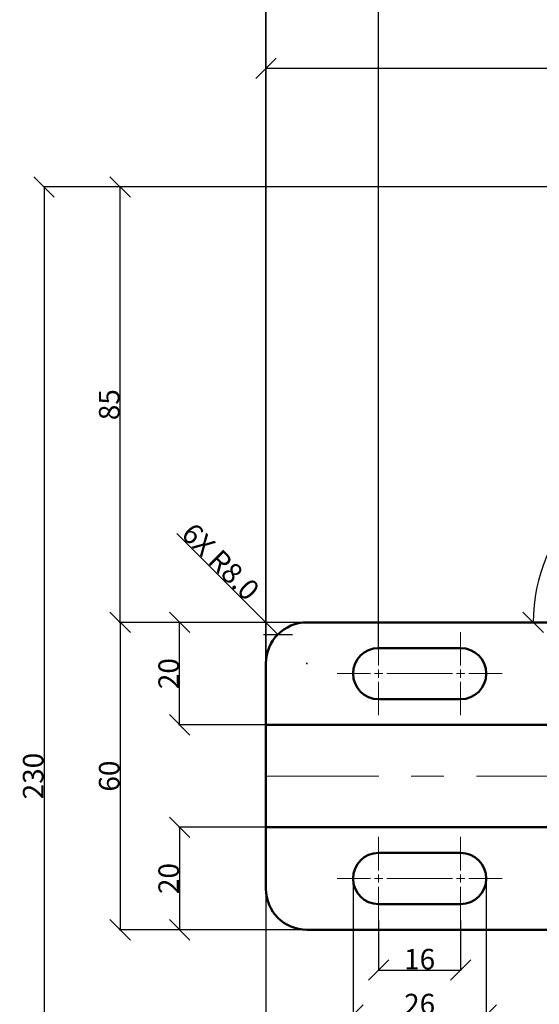
# Model space of a CAD drawing. Units: millimetres. Extents: x 263 to 611, y 50 to 522.
# Tile 2 of 5: x 263 to 364, y 157 to 349. Entities that reach past the tile are written whole.
import ezdxf

# ---------------------------------------------------------------- set-up
doc = ezdxf.new("R2010")
doc.units = ezdxf.units.MM
doc.header["$MEASUREMENT"] = 0
doc.linetypes.add('CENTER', pattern=[50.8, 31.75, -6.35, 6.35, -6.35])
for name, color, linetype, lineweight in [('M-CNTR', 1, 'CENTER', 18), ('M-DIMS', 2, 'Continuous', 25), ('M-OUTL', 7, 'Continuous', 50)]:
    doc.layers.add(name, color=color, linetype=linetype, lineweight=lineweight)
doc.styles.get("Standard").update_dxf_attribs({"font": 'arial.ttf'})
doc.dimstyles.get("Standard").update_dxf_attribs({"dimtxt": 4, "dimasz": 4, "dimexe": 0.18, "dimexo": 0.0625, "dimgap": 0.09, "dimtad": 1, "dimdec": 0, "dimzin": 0, "dimdsep": 46, "dimtxsty": 'Standard', "dimblk": 'OBLIQUE', "dimcen": 0.09, "dimclre": 251, "dimadec": 0, "dimazin": 0, "dimtfac": 1, "dimtdec": 0, "dimtofl": 0, "dimtmove": 0, "dimatfit": 3, "dimfxl": 1, "dimtolj": 1, "dimtzin": 0, "dimarcsym": 0})

# ---------------------------------------------------------------- blocks, each defined once
blk = doc.blocks.new('_Oblique')
at = {"color": 0, "linetype": 'ByBlock', "lineweight": -2}
blk.add_line((-0.5, -0.5), (0.5, 0.5), dxfattribs=at)
blk = doc.blocks.new('*D5')
at = {"layer": 'Defpoints', "color": 0, "transparency": 16777216}
for p in [(319.1, 231.08), (282.64, 171.08), (319.1, 171.08)]:
    blk.add_point(p, dxfattribs=at)
at = {"layer": 'M-DIMS', "color": 0, "lineweight": -2, "transparency": 16777216}
for p, q in [((319.04, 231.08), (282.46, 231.08)), ((282.64, 231.08), (282.64, 171.08)), ((319.04, 171.08), (282.46, 171.08))]:
    blk.add_line(p, q, dxfattribs=at)
at = {"layer": 'M-DIMS', "color": 0, "lineweight": -2, "transparency": 16777216, "xscale": 4, "yscale": 4, "zscale": 4}
for p, rotation in [((282.64, 231.08), 90), ((282.64, 171.08), 270)]:
    blk.add_blockref('_Oblique', p, dxfattribs=dict(at, rotation=rotation))
at = {"layer": 'M-DIMS', "color": 0, "transparency": 16777216, "insert": (280.51, 201.08), "char_height": 4, "attachment_point": 5, "rotation": 90}
blk.add_mtext('\\A1;60', dxfattribs=at)
blk = doc.blocks.new('*U6')
at = {"layer": 'M-CNTR', "color": 0, "transparency": 16777216}
for p, q in [((0, 1.6), (0, 8.12)), ((-8.12, 0), (-1.6, 0)), ((1.6, 0), (8.12, 0)), ((0, -8.12), (0, -1.6))]:
    blk.add_line(p, q, dxfattribs=at)
at = {"layer": 'M-CNTR', "color": 0, "linetype": 'Continuous', "transparency": 16777216}
for p, q in [((-0.8, 0), (0.8, 0)), ((0, -0.8), (0, 0.8))]:
    blk.add_line(p, q, dxfattribs=at)
blk = doc.blocks.new('*U7')
at = {"layer": 'M-CNTR', "color": 0, "transparency": 16777216}
for p, q in [((0, 1.6), (0, 8.12)), ((-8.12, 0), (-1.6, 0)), ((1.6, 0), (8.12, 0)), ((0, -8.12), (0, -1.6))]:
    blk.add_line(p, q, dxfattribs=at)
at = {"layer": 'M-CNTR', "color": 0, "linetype": 'Continuous', "transparency": 16777216}
for p, q in [((-0.8, 0), (0.8, 0)), ((0, -0.8), (0, 0.8))]:
    blk.add_line(p, q, dxfattribs=at)
blk = doc.blocks.new('*U8')
at = {"layer": 'M-CNTR', "color": 0, "transparency": 16777216}
for p, q in [((0, 1.6), (0, 8.12)), ((-8.12, 0), (-1.6, 0)), ((1.6, 0), (8.12, 0)), ((0, -8.12), (0, -1.6))]:
    blk.add_line(p, q, dxfattribs=at)
at = {"layer": 'M-CNTR', "color": 0, "linetype": 'Continuous', "transparency": 16777216}
for p, q in [((-0.8, 0), (0.8, 0)), ((0, -0.8), (0, 0.8))]:
    blk.add_line(p, q, dxfattribs=at)
blk = doc.blocks.new('*U9')
at = {"layer": 'M-CNTR', "color": 0, "transparency": 16777216}
for p, q in [((0, 1.6), (0, 8.12)), ((-8.12, 0), (-1.6, 0)), ((1.6, 0), (8.12, 0)), ((0, -8.12), (0, -1.6))]:
    blk.add_line(p, q, dxfattribs=at)
at = {"layer": 'M-CNTR', "color": 0, "linetype": 'Continuous', "transparency": 16777216}
for p, q in [((-0.8, 0), (0.8, 0)), ((0, -0.8), (0, 0.8))]:
    blk.add_line(p, q, dxfattribs=at)
blk = doc.blocks.new('*D18')
at = {"layer": 'Defpoints', "color": 0, "transparency": 16777216}
for p in [(546.1, 339.25), (546.1, 231.08), (311.1, 223.08)]:
    blk.add_point(p, dxfattribs=at)
at = {"layer": 'M-DIMS', "color": 0, "lineweight": -2, "transparency": 16777216}
for p, q in [((311.1, 223.14), (311.1, 339.43)), ((311.1, 339.25), (546.1, 339.25)), ((546.1, 231.14), (546.1, 339.43))]:
    blk.add_line(p, q, dxfattribs=at)
at = {"layer": 'M-DIMS', "color": 0, "lineweight": -2, "transparency": 16777216, "xscale": 4, "yscale": 4, "zscale": 4, "rotation": 180}
blk.add_blockref('_Oblique', (311.1, 339.25), dxfattribs=at)
at = {"layer": 'M-DIMS', "color": 0, "lineweight": -2, "transparency": 16777216, "xscale": 4, "yscale": 4, "zscale": 4}
blk.add_blockref('_Oblique', (546.1, 339.25), dxfattribs=at)
at = {"layer": 'M-DIMS', "color": 0, "transparency": 16777216, "insert": (428.6, 341.39), "char_height": 4, "attachment_point": 5}
blk.add_mtext('\\A1;235', dxfattribs=at)
blk = doc.blocks.new('*D19')
at = {"layer": 'Defpoints', "color": 0, "transparency": 16777216}
for p in [(294.25, 231.08), (319.1, 231.08), (311.1, 211.08)]:
    blk.add_point(p, dxfattribs=at)
at = {"layer": 'M-DIMS', "color": 0, "lineweight": -2, "transparency": 16777216}
for p, q in [((319.04, 231.08), (294.07, 231.08)), ((294.25, 211.08), (294.25, 231.08)), ((311.04, 211.08), (294.07, 211.08))]:
    blk.add_line(p, q, dxfattribs=at)
at = {"layer": 'M-DIMS', "color": 0, "lineweight": -2, "transparency": 16777216, "xscale": 4, "yscale": 4, "zscale": 4}
for p, rotation in [((294.25, 231.08), 90), ((294.25, 211.08), 270)]:
    blk.add_blockref('_Oblique', p, dxfattribs=dict(at, rotation=rotation))
at = {"layer": 'M-DIMS', "color": 0, "transparency": 16777216, "insert": (292.12, 221.08), "char_height": 4, "attachment_point": 5, "rotation": 90}
blk.add_mtext('\\A1;20', dxfattribs=at)
blk = doc.blocks.new('*D20')
at = {"layer": 'Defpoints', "color": 0, "transparency": 16777216}
for p in [(311.1, 191.08), (294.25, 171.08), (319.1, 171.08)]:
    blk.add_point(p, dxfattribs=at)
at = {"layer": 'M-DIMS', "color": 0, "lineweight": -2, "transparency": 16777216}
for p, q in [((311.04, 191.08), (294.07, 191.08)), ((294.25, 191.08), (294.25, 171.08)), ((319.04, 171.08), (294.07, 171.08))]:
    blk.add_line(p, q, dxfattribs=at)
at = {"layer": 'M-DIMS', "color": 0, "lineweight": -2, "transparency": 16777216, "xscale": 4, "yscale": 4, "zscale": 4}
for p, rotation in [((294.25, 191.08), 90), ((294.25, 171.08), 270)]:
    blk.add_blockref('_Oblique', p, dxfattribs=dict(at, rotation=rotation))
at = {"layer": 'M-DIMS', "color": 0, "transparency": 16777216, "insert": (292.12, 181.08), "char_height": 4, "attachment_point": 5, "rotation": 90}
blk.add_mtext('\\A1;20', dxfattribs=at)
blk = doc.blocks.new('*D21')
at = {"layer": 'Defpoints', "color": 0, "transparency": 16777216}
for p in [(282.64, 316.08), (404.1, 316.08), (319.1, 231.08)]:
    blk.add_point(p, dxfattribs=at)
at = {"layer": 'M-DIMS', "color": 0, "lineweight": -2, "transparency": 16777216}
for p, q in [((404.04, 316.08), (282.46, 316.08)), ((282.64, 231.08), (282.64, 316.08)), ((319.04, 231.08), (282.46, 231.08))]:
    blk.add_line(p, q, dxfattribs=at)
at = {"layer": 'M-DIMS', "color": 0, "lineweight": -2, "transparency": 16777216, "xscale": 4, "yscale": 4, "zscale": 4}
for p, rotation in [((282.64, 316.08), 90), ((282.64, 231.08), 270)]:
    blk.add_blockref('_Oblique', p, dxfattribs=dict(at, rotation=rotation))
at = {"layer": 'M-DIMS', "color": 0, "transparency": 16777216, "insert": (280.51, 273.58), "char_height": 4, "attachment_point": 5, "rotation": 90}
blk.add_mtext('\\A1;85', dxfattribs=at)
blk = doc.blocks.new('*D22')
at = {"layer": 'Defpoints', "color": 0, "transparency": 16777216}
for p in [(404.1, 316.08), (267.8, 86.08), (404.1, 86.08)]:
    blk.add_point(p, dxfattribs=at)
at = {"layer": 'M-DIMS', "color": 0, "lineweight": -2, "transparency": 16777216}
for p, q in [((404.04, 316.08), (267.62, 316.08)), ((267.8, 316.08), (267.8, 86.08)), ((404.04, 86.08), (267.62, 86.08))]:
    blk.add_line(p, q, dxfattribs=at)
at = {"layer": 'M-DIMS', "color": 0, "lineweight": -2, "transparency": 16777216, "xscale": 4, "yscale": 4, "zscale": 4}
for p, rotation in [((267.8, 316.08), 90), ((267.8, 86.08), 270)]:
    blk.add_blockref('_Oblique', p, dxfattribs=dict(at, rotation=rotation))
at = {"layer": 'M-DIMS', "color": 0, "transparency": 16777216, "insert": (265.67, 201.08), "char_height": 4, "attachment_point": 5, "rotation": 90}
blk.add_mtext('\\A1;230', dxfattribs=at)
blk = doc.blocks.new('*D23')
at = {"layer": 'Defpoints', "color": 0, "transparency": 16777216}
for p in [(333.1, 172.96), (349.1, 172.96), (349.1, 163.22)]:
    blk.add_point(p, dxfattribs=at)
at = {"layer": 'M-DIMS', "color": 0, "lineweight": -2, "transparency": 16777216}
for p, q in [((333.1, 172.9), (333.1, 163.04)), ((349.1, 172.9), (349.1, 163.04)), ((333.1, 163.22), (349.1, 163.22))]:
    blk.add_line(p, q, dxfattribs=at)
at = {"layer": 'M-DIMS', "color": 0, "lineweight": -2, "transparency": 16777216, "xscale": 4, "yscale": 4, "zscale": 4, "rotation": 180}
blk.add_blockref('_Oblique', (333.1, 163.22), dxfattribs=at)
at = {"layer": 'M-DIMS', "color": 0, "lineweight": -2, "transparency": 16777216, "xscale": 4, "yscale": 4, "zscale": 4}
blk.add_blockref('_Oblique', (349.1, 163.22), dxfattribs=at)
at = {"layer": 'M-DIMS', "color": 0, "transparency": 16777216, "insert": (341.1, 165.35), "char_height": 4, "attachment_point": 5}
blk.add_mtext('\\A1;16', dxfattribs=at)
blk = doc.blocks.new('*D24')
at = {"layer": 'Defpoints', "color": 0, "transparency": 16777216}
for p in [(328.1, 181.08), (354.1, 181.08), (354.1, 154.45)]:
    blk.add_point(p, dxfattribs=at)
at = {"layer": 'M-DIMS', "color": 0, "lineweight": -2, "transparency": 16777216}
for p, q in [((328.1, 181.02), (328.1, 154.27)), ((354.1, 181.02), (354.1, 154.27)), ((328.1, 154.45), (354.1, 154.45))]:
    blk.add_line(p, q, dxfattribs=at)
at = {"layer": 'M-DIMS', "color": 0, "lineweight": -2, "transparency": 16777216, "xscale": 4, "yscale": 4, "zscale": 4, "rotation": 180}
blk.add_blockref('_Oblique', (328.1, 154.45), dxfattribs=at)
at = {"layer": 'M-DIMS', "color": 0, "lineweight": -2, "transparency": 16777216, "xscale": 4, "yscale": 4, "zscale": 4}
blk.add_blockref('_Oblique', (354.1, 154.45), dxfattribs=at)
at = {"layer": 'M-DIMS', "color": 0, "transparency": 16777216, "insert": (341.1, 156.58), "char_height": 4, "attachment_point": 5}
blk.add_mtext('\\A1;26', dxfattribs=at)
blk = doc.blocks.new('*D25')
at = {"layer": 'Defpoints', "color": 0, "transparency": 16777216}
for p in [(311.1, 201.08), (426.1, 201.08), (426.1, 140.57)]:
    blk.add_point(p, dxfattribs=at)
at = {"layer": 'M-DIMS', "color": 0, "lineweight": -2, "transparency": 16777216}
for p, q in [((311.1, 201.02), (311.1, 140.39)), ((426.1, 201.02), (426.1, 140.39)), ((311.1, 140.57), (426.1, 140.57))]:
    blk.add_line(p, q, dxfattribs=at)
at = {"layer": 'M-DIMS', "color": 0, "lineweight": -2, "transparency": 16777216, "xscale": 4, "yscale": 4, "zscale": 4, "rotation": 180}
blk.add_blockref('_Oblique', (311.1, 140.57), dxfattribs=at)
at = {"layer": 'M-DIMS', "color": 0, "lineweight": -2, "transparency": 16777216, "xscale": 4, "yscale": 4, "zscale": 4}
blk.add_blockref('_Oblique', (426.1, 140.57), dxfattribs=at)
at = {"layer": 'M-DIMS', "color": 0, "transparency": 16777216, "insert": (368.6, 142.7), "char_height": 4, "attachment_point": 5}
blk.add_mtext('\\A1;115', dxfattribs=at)
blk = doc.blocks.new('*D29')
at = {"layer": 'Defpoints', "color": 0, "transparency": 16777216}
for p in [(396.1, 308.08), (379.68, 259.52), (396.1, 247.18), (319.1, 231.08), (380, 231.08)]:
    blk.add_point(p, dxfattribs=at)
at = {"layer": 'M-DIMS', "color": 0, "lineweight": -2, "transparency": 16777216}
blk.add_arc((396.1, 231.08), 32.84, 90, 180, dxfattribs=at)
at = {"layer": 'M-DIMS', "color": 0, "lineweight": -2, "transparency": 16777216, "xscale": 4, "yscale": 4, "zscale": 4}
for p, rotation in [((396.1, 263.92), 359.9999999999999), ((363.26, 231.08), 269.9999999999999)]:
    blk.add_blockref('_Oblique', p, dxfattribs=dict(at, rotation=rotation))
at = {"layer": 'M-DIMS', "color": 0, "transparency": 16777216, "insert": (371.37, 255.81), "char_height": 4, "attachment_point": 5, "rotation": 45}
blk.add_mtext('\\A1;90°', dxfattribs=at)
blk = doc.blocks.new('SLOT-10x26')
for p, q in [((0, 5), (0, 21)), ((10, 5), (10, 21))]:
    blk.add_line(p, q)
for centre, start, end in [((5, 21), 0, 180), ((5, 5), 180, 0)]:
    blk.add_arc(centre, 5, start, end)
blk = doc.blocks.new('*D52')
at = {"layer": 'Defpoints', "color": 0, "transparency": 16777216}
for p in [(333.1, 517.18), (333.1, 226.08), (311.1, 223.08)]:
    blk.add_point(p, dxfattribs=at)
at = {"layer": 'M-DIMS', "color": 251, "lineweight": -2, "transparency": 16777216}
for p, q in [((311.1, 223.14), (311.1, 517.36)), ((333.1, 226.14), (333.1, 517.36))]:
    blk.add_line(p, q, dxfattribs=at)
at = {"layer": 'M-DIMS', "color": 0, "lineweight": -2, "transparency": 16777216}
blk.add_line((311.1, 517.18), (333.1, 517.18), dxfattribs=at)
at = {"layer": 'M-DIMS', "color": 0, "lineweight": -2, "transparency": 16777216, "xscale": 4, "yscale": 4, "zscale": 4, "rotation": 180}
blk.add_blockref('_Oblique', (311.1, 517.18), dxfattribs=at)
at = {"layer": 'M-DIMS', "color": 0, "lineweight": -2, "transparency": 16777216, "xscale": 4, "yscale": 4, "zscale": 4}
blk.add_blockref('_Oblique', (333.1, 517.18), dxfattribs=at)
at = {"layer": 'M-DIMS', "color": 0, "transparency": 16777216, "insert": (322.1, 519.31), "char_height": 4, "attachment_point": 5}
blk.add_mtext('\\A1;22.0', dxfattribs=at)
blk = doc.blocks.new('*D53')
at = {"layer": 'Defpoints', "color": 0, "transparency": 16777216}
for p in [(578.1, 423.27), (311.1, 383.27), (578.1, 52.26)]:
    blk.add_point(p, dxfattribs=at)
at = {"layer": 'M-DIMS', "color": 251, "lineweight": -2, "transparency": 16777216}
for p, q in [((578.1, 423.21), (578.1, 52.08)), ((311.1, 383.21), (311.1, 52.08))]:
    blk.add_line(p, q, dxfattribs=at)
at = {"layer": 'M-DIMS', "color": 0, "lineweight": -2, "transparency": 16777216}
blk.add_line((311.1, 52.26), (578.1, 52.26), dxfattribs=at)
at = {"layer": 'M-DIMS', "color": 0, "lineweight": -2, "transparency": 16777216, "xscale": 4, "yscale": 4, "zscale": 4, "rotation": 180}
blk.add_blockref('_Oblique', (311.1, 52.26), dxfattribs=at)
at = {"layer": 'M-DIMS', "color": 0, "lineweight": -2, "transparency": 16777216, "xscale": 4, "yscale": 4, "zscale": 4}
blk.add_blockref('_Oblique', (578.1, 52.26), dxfattribs=at)
at = {"layer": 'M-DIMS', "color": 0, "transparency": 16777216, "insert": (444.6, 54.39), "char_height": 4, "attachment_point": 5}
blk.add_mtext('\\A1;267.0', dxfattribs=at)
blk = doc.blocks.new('*D57')
at = {"layer": 'Defpoints', "color": 0, "transparency": 16777216}
for p in [(372.02, 403.27), (311.1, 383.27), (372.02, 52.26)]:
    blk.add_point(p, dxfattribs=at)
at = {"layer": 'M-DIMS', "color": 251, "lineweight": -2, "transparency": 16777216}
for p, q in [((372.02, 403.21), (372.02, 52.08)), ((311.1, 383.21), (311.1, 52.08))]:
    blk.add_line(p, q, dxfattribs=at)
at = {"layer": 'M-DIMS', "color": 0, "lineweight": -2, "transparency": 16777216}
blk.add_line((311.1, 52.26), (372.02, 52.26), dxfattribs=at)
at = {"layer": 'M-DIMS', "color": 0, "lineweight": -2, "transparency": 16777216, "xscale": 4, "yscale": 4, "zscale": 4, "rotation": 180}
blk.add_blockref('_Oblique', (311.1, 52.26), dxfattribs=at)
at = {"layer": 'M-DIMS', "color": 0, "lineweight": -2, "transparency": 16777216, "xscale": 4, "yscale": 4, "zscale": 4}
blk.add_blockref('_Oblique', (372.02, 52.26), dxfattribs=at)
at = {"layer": 'M-DIMS', "color": 0, "transparency": 16777216, "insert": (341.56, 54.39), "char_height": 4, "attachment_point": 5}
blk.add_mtext('\\A1;60.92', dxfattribs=at)
blk = doc.blocks.new('*D69')
at = {"layer": 'Defpoints', "color": 0, "transparency": 16777216}
for p in [(426.1, 201.08), (387.21, 162.19)]:
    blk.add_point(p, dxfattribs=at)
at = {"layer": 'M-DIMS', "color": 251, "lineweight": -2, "transparency": 16777216}
for p, q in [((426.01, 201.08), (426.19, 201.08)), ((426.1, 200.99), (426.1, 201.17))]:
    blk.add_line(p, q, dxfattribs=at)
at = {"layer": 'M-DIMS', "color": 0, "lineweight": -2, "transparency": 16777216}
blk.add_line((355.69, 130.68), (387.21, 162.19), dxfattribs=at)
at = {"layer": 'M-DIMS', "color": 0, "lineweight": -2, "transparency": 16777216, "xscale": 4, "yscale": 4, "zscale": 4, "rotation": 44.99977533015295}
blk.add_blockref('_Oblique', (387.21, 162.19), dxfattribs=at)
at = {"layer": 'M-DIMS', "color": 0, "transparency": 16777216, "insert": (362.37, 140.36), "char_height": 4, "attachment_point": 5, "rotation": 44.9998}
blk.add_mtext('\\A1;4X R55.0', dxfattribs=at)
blk = doc.blocks.new('*D80')
at = {"layer": 'Defpoints', "color": 0, "transparency": 16777216}
for p in [(313.44, 228.74), (319.1, 223.08)]:
    blk.add_point(p, dxfattribs=at)
at = {"layer": 'M-DIMS', "color": 0, "lineweight": -2, "transparency": 16777216}
blk.add_line((293.72, 248.46), (313.44, 228.74), dxfattribs=at)
at = {"layer": 'M-DIMS', "color": 251, "lineweight": -2, "transparency": 16777216}
for p, q in [((319.01, 223.08), (319.19, 223.08)), ((319.1, 222.99), (319.1, 223.17))]:
    blk.add_line(p, q, dxfattribs=at)
at = {"layer": 'M-DIMS', "color": 0, "lineweight": -2, "transparency": 16777216, "xscale": 4, "yscale": 4, "zscale": 4, "rotation": 315.001848461854}
blk.add_blockref('_Oblique', (313.44, 228.74), dxfattribs=at)
at = {"layer": 'M-DIMS', "color": 0, "transparency": 16777216, "insert": (302.26, 242.94), "char_height": 4, "attachment_point": 5, "rotation": 315.0018}
blk.add_mtext('\\A1;6X R8.0', dxfattribs=at)

msp = doc.modelspace()

# ---------------------------------------------------------------- linework, layer by layer
at = {"layer": 'M-CNTR'}
msp.add_line((587.1329, 201.0815), (311.0988, 201.0815), dxfattribs=at)
at = {"layer": 'M-OUTL'}
for p, q in [((319.0988, 231.0815), (380.0011, 231.0815)), ((311.0988, 179.0815), (311.0988, 223.0815)), ((311.0988, 211.0815), (372.0156, 211.0815)), ((311.0988, 191.0815), (372.0156, 191.0815)), ((319.0988, 171.0815), (380.0011, 171.0815))]:
    msp.add_line(p, q, dxfattribs=at)
for centre, start, end in [((319.0988, 223.0815), 90, 180), ((319.0988, 179.0815), 180, 270)]:
    msp.add_arc(centre, 8, start, end, dxfattribs=at)

# ---------------------------------------------------------------- block references
at = {"layer": 'M-CNTR'}
for name, p in [('*U6', (333.0988, 221.0815)), ('*U7', (349.0988, 221.0815)), ('*U8', (333.0988, 181.0815)), ('*U9', (349.0988, 181.0815))]:
    msp.add_blockref(name, p, dxfattribs=at)
at = {"layer": 'M-OUTL'}
for p, rotation in [((328.0993, 226.0814), 269.9999999999999), ((328.0993, 186.0814), 269.9999999999998)]:
    msp.add_blockref('SLOT-10x26', p, dxfattribs=dict(at, rotation=rotation))

# ---------------------------------------------------------------- dimensions: what is measured, and where the dimension line sits
at = {"layer": 'M-DIMS'}
for base, p1, p2, override, picture, middle in [((333.0988, 517.1806), (311.0988, 223.0815), (333.0988, 226.0815), {"dimdec": 1, "dimlfac": 1, "dimrnd": 0, "dimzin": 0, "dimdsep": 46, "dimlunit": 2}, '*D52', (322.0988, 519.3128)), ((578.0988, 52.2557), (311.0988, 383.2727), (578.0988, 423.2727), {"dimdec": 1, "dimlfac": 1, "dimrnd": 0, "dimzin": 0, "dimdsep": 46, "dimlunit": 2}, '*D53', (444.5988, 54.388)), ((372.0156, 52.2557), (311.0988, 383.2727), (372.0156, 403.2727), {"dimdec": 2, "dimlfac": 1, "dimrnd": 0, "dimzin": 0, "dimdsep": 46, "dimlunit": 2}, '*D57', (341.5572, 54.388)), ((546.0988, 339.2528), (311.0988, 223.0815), (546.0988, 231.0815), {"dimclrd": 0, "dimclre": 0, "dimclrt": 0}, '*D18', (428.5988, 341.3864)), ((426.0988, 140.5664), (311.0988, 201.0815), (426.0988, 201.0815), {"dimclrd": 0, "dimclre": 0, "dimclrt": 0}, '*D25', (368.5988, 142.6987)), ((354.0988, 154.4515), (328.0988, 181.0815), (354.0988, 181.0815), {"dimclrd": 0, "dimclre": 0, "dimclrt": 0}, '*D24', (341.0988, 156.5838)), ((349.0988, 163.215), (333.0988, 172.9615), (349.0988, 172.9615), {"dimclrd": 0, "dimclre": 0, "dimclrt": 0}, '*D23', (341.0988, 165.3473))]:
    dim = msp.add_linear_dim(base=base, p1=p1, p2=p2, dimstyle='Standard', override=override, dxfattribs=at)
    dim.commit()
    dim.dimension.update_dxf_attribs({"geometry": picture, "text_midpoint": middle})
for base, p1, p2, picture, middle in [((267.7992, 86.0815), (404.0988, 316.0815), (404.0988, 86.0815), '*D22', (265.6656, 201.0815)), ((282.6439, 316.0815), (319.0988, 231.0815), (404.0988, 316.0815), '*D21', (280.5117, 273.5815)), ((282.6439, 171.0815), (319.0988, 231.0815), (319.0988, 171.0815), '*D5', (280.5117, 201.0815)), ((294.2541, 231.0815), (311.0988, 211.0815), (319.0988, 231.0815), '*D19', (292.1219, 221.0815)), ((294.2541, 171.0815), (311.0988, 191.0815), (319.0988, 171.0815), '*D20', (292.1219, 181.0815))]:
    dim = msp.add_linear_dim(base=base, p1=p1, p2=p2, angle=90, dimstyle='Standard', override={"dimclrd": 0, "dimclre": 0, "dimclrt": 0}, dxfattribs=at)
    dim.commit()
    dim.dimension.update_dxf_attribs({"geometry": picture, "text_midpoint": middle})
dim = msp.add_angular_dim_2l(base=(379.6771, 259.5248), line1=((396.0988, 308.0815), (396.0988, 247.1793)), line2=((319.0988, 231.0815), (380.0011, 231.0815)), dimstyle='Standard', override={"dimclrd": 0, "dimclre": 0, "dimclrt": 0}, dxfattribs=at)
dim.commit()
dim.dimension.update_dxf_attribs({"geometry": '*D29', "text_midpoint": (371.3673, 255.8131)})
dim = msp.add_radius_dim(center=(319.0988, 223.0815), mpoint=(313.4418, 228.7382), text='6X <>', dimstyle='Standard', override={"dimdec": 1, "dimlfac": 1, "dimrnd": 0, "dimzin": 0, "dimdsep": 46, "dimlunit": 2}, dxfattribs=at)
dim.commit()
dim.dimension.update_dxf_attribs({"geometry": '*D80', "text_midpoint": (302.2588, 242.9359)})
dim = msp.add_radius_dim(center=(426.0988, 201.0815), mpoint=(387.2078, 162.1908), text='4X <>', dimstyle='Standard', override={"dimdec": 1, "dimlfac": 1, "dimrnd": 0, "dimzin": 0, "dimdsep": 46, "dimlunit": 2}, dxfattribs=at)
dim.commit()
dim.dimension.update_dxf_attribs({"geometry": '*D69', "text_midpoint": (363.8732, 138.8564), "dimtype": 164})

doc.saveas('drawing.dxf')
